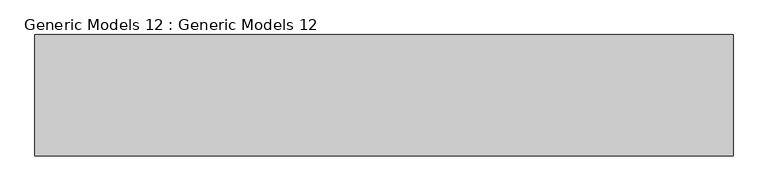
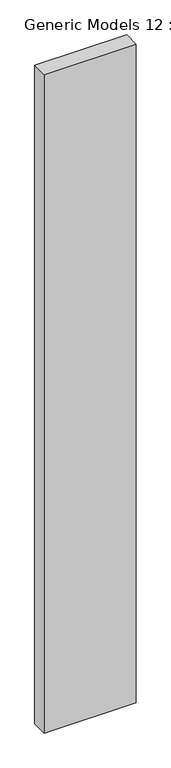
"""IFC4 building model written with IfcOpenShell, lengths in millimetres: proxy geometry, Generic Models 12 : Generic Models 12."""

from ifc_helpers import new_model, si_unit, frame, origin, place, context, project, spatial, polyline, outline, extrude, source, transform, mapped, element, save


def generic_models_12_generic_models_12_a991e301(model_context):
    return source(origin(), model_context, "Body", "SweptSolid", [
        extrude(outline(polyline([(9809.3020354, -3746.0004242), (9809.3020354, -4404.8405988), (6019.3116921, -4404.8405988), (6019.3116921, -3746.0004242), (9809.3020354, -3746.0004242)])), frame((0.0, 0.0, 3411.9703205), z_axis=(0.0, 0.0, 1.0), x_axis=(1.0, 0.0, 0.0)), (0.0, 0.0, 1.0), 28648.0304545),
    ])


if __name__ == "__main__":
    model = new_model("IFC4")
    model_context = context("Model", 3, world=origin())
    ifc_project = project(units=[si_unit("LENGTHUNIT", "METRE", prefix="MILLI")], contexts=[model_context])
    site = spatial("IfcSite", under=ifc_project)
    building = spatial("IfcBuilding", under=site)
    placement = place(None, origin())
    generic_models_12_generic_models_12_shape = generic_models_12_generic_models_12_a991e301(model_context)
    element("IfcBuildingElementProxy", 1, Name="Generic Models 12 : Generic Models 12", ObjectType="Generic Models 12 : Generic Models 12", at=placement, inside=building, context=model_context, shape_type="MappedRepresentation", body=[
        mapped(generic_models_12_generic_models_12_shape, transform((0.0, 0.0, 0.0), x_axis=(1.0, 0.0, 0.0), y_axis=(0.0, 1.0, 0.0), z_axis=(0.0, 0.0, 1.0))),
    ])
    save(model, "model.ifc")
